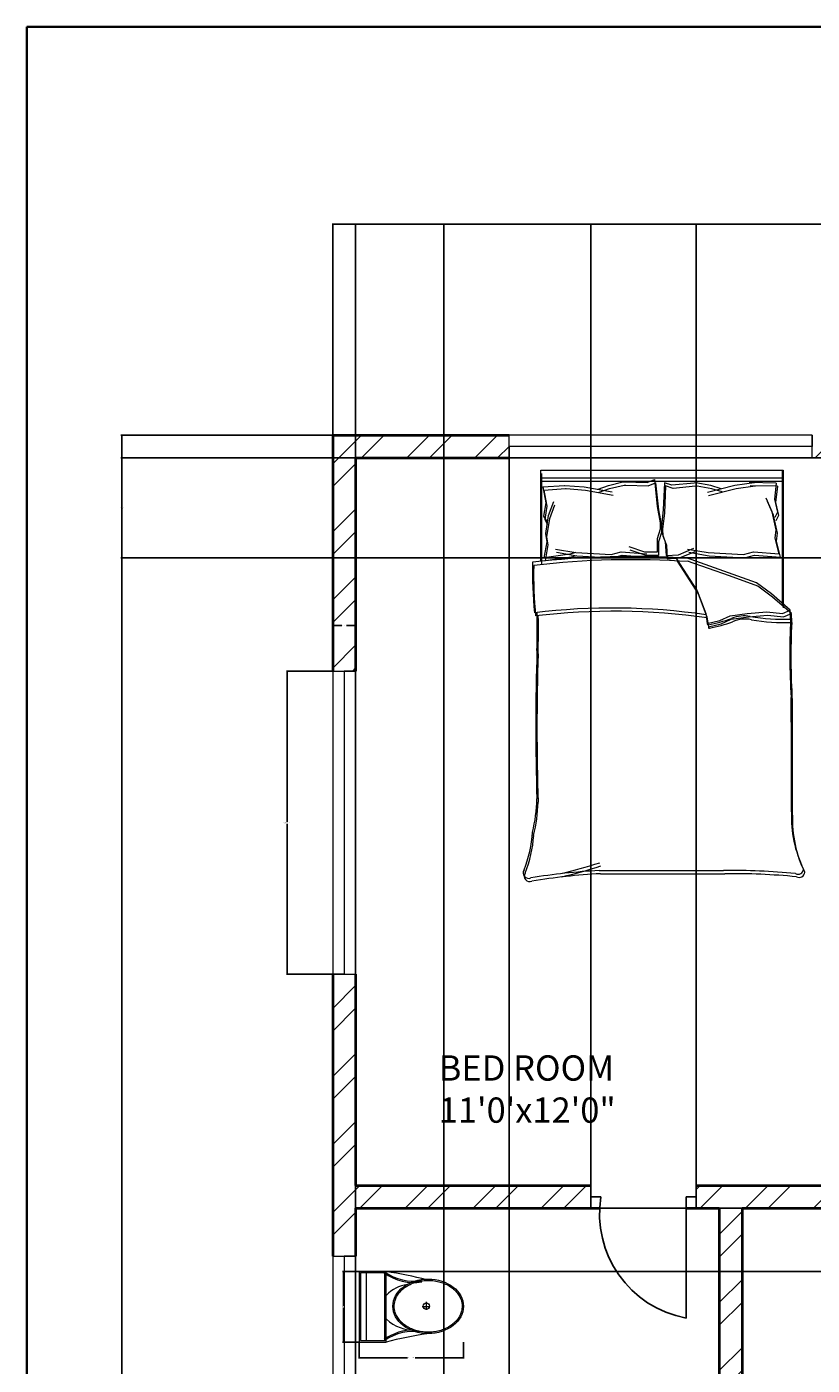
# Model space of a CAD drawing. Units: inches. Extents: x 2063 to 2617, y 1299 to 2210.
# Tile 13 of 22: x 2063 to 2218, y 1945 to 2210. Entities that reach past the tile are written whole.
import ezdxf

# ---------------------------------------------------------------- set-up
doc = ezdxf.new("R2010")
doc.units = ezdxf.units.IN
for name, color, linetype, lineweight in [('A-ANNO-DIMS', 2, 'Continuous', 18), ('A-ANNO-TTLB', 7, 'Continuous', 35), ('A-AREA-IDEN', 7, 'Continuous', 18), ('A-DOOR', 11, 'Continuous', 25), ('A-FLOR-FIXT', 8, 'Continuous', 18), ('A-FURN', 8, 'Continuous', 18), ('A-GLAZ', 123, 'Continuous', 18), ('A-WALL', 7, 'Continuous', 40)]:
    doc.layers.add(name, color=color, linetype=linetype, lineweight=lineweight)
doc.layers.add('A-WALL-PATT', color=215, linetype='Continuous', lineweight=13, true_color=0xa953a0)
doc.styles.get("Standard").update_dxf_attribs({"font": 'arial.ttf'})
doc.dimstyles.get("Standard").update_dxf_attribs({"dimtxt": 0.18, "dimasz": 0.18, "dimexe": 0.18, "dimexo": 0.0625, "dimgap": 0.09, "dimtad": 0, "dimtih": 1, "dimtoh": 1, "dimdec": 4, "dimzin": 0, "dimdsep": 46, "dimtxsty": 'Standard', "dimcen": 0.09, "dimadec": 0, "dimazin": 0, "dimtfac": 1, "dimtdec": 4, "dimtofl": 0, "dimtmove": 0, "dimatfit": 3, "dimfxl": 1, "dimtolj": 1, "dimtzin": 0, "dimarcsym": 0})

# ---------------------------------------------------------------- blocks, each defined once
blk = doc.blocks.new('A$C31115884')
for p, q in [((283.1, 497.7), (223.4, 497.7)), ((257.5, 466.4), (257.5, 523.2)), ((0, 200), (0, 0)), ((520, 200), (0, 200)), ((520, 0), (520, 200)), ((10, 190), (10, 10)), ((510, 190), (10, 190)), ((510, 10), (510, 190)), ((510, 54.5), (0, 54.5)), ((10, 10), (510, 10)), ((0, 0), (520, 0))]:
    blk.add_line(p, q)
blk.add_circle((255.6, 496.4), 23.6)
for centre, radius, start, end in [((2777.7, -204.6), 2807, 165.4549, 171.71327), ((3237, 905), 2807, 188.28673, 194.5451), ((-294.5, 403.3), 364.7, 324.20913, 9.34987), ((-294.5, 403.3), 374.7, 324.20913, 9.34987), ((139.5, 406.2), 293.5, 315.84364, 2.65635), ((805.8, 403.3), 374.7, 179.20365, 215.79087), ((805.8, 403.3), 364.7, 170.65013, 215.79087), ((383.6, 406.2), 293.5, 190.27735, 224.15636)]:
    blk.add_arc(centre, radius, start, end)
blk.add_ellipse((256.2, 509.9), major_axis=(0, -260.7), ratio=0.772727)
blk.add_open_spline([(256.2, 259.2), (263.1, 259.2), (270, 259.7), (287.8, 262.3), (298.7, 265.1), (319.9, 273.1), (330.2, 278.4), (350.1, 291.1), (359.7, 298.7), (377.7, 315.9), (386.2, 325.5), (401.7, 346.6), (408.8, 358.1), (421.3, 382.5), (426.8, 395.5), (435.9, 422.4), (439.5, 436.4), (444.8, 465.1), (446.5, 479.7), (447.9, 509.2), (447.6, 524), (445, 553.3), (442.7, 567.8), (436.3, 596), (432.1, 609.7), (421.9, 636), (416, 648.6), (402.5, 672.1), (395, 683), (378.6, 703), (369.8, 712.1), (351.1, 728), (341.3, 734.8), (320.9, 746.2), (310.4, 750.7), (288.9, 757.3), (278, 759.4), (256, 761), (245, 760.6), (223.1, 757.2), (212.3, 754.3), (191.1, 746.1), (180.8, 740.7), (160.9, 727.8), (151.4, 720.1), (133.5, 702.7), (125.1, 693), (109.6, 671.7), (102.6, 660.2), (90.2, 635.7), (84.9, 622.7), (76, 595.6), (72.4, 581.6), (67.2, 552.9), (65.6, 538.2), (64.4, 508.8), (64.8, 494), (67.5, 464.7), (69.9, 450.2), (76.6, 422), (80.8, 408.3), (91.1, 382.2), (97.2, 369.7), (110.8, 346.3), (118.4, 335.4), (134.8, 315.6), (143.7, 306.7), (162.4, 290.9), (172.3, 284.2), (192.8, 273), (203.3, 268.6), (224.8, 262.2), (235.8, 260.2), (249.9, 259.3), (253, 259.2), (256.2, 259.2)], degree=3, knots=[0, 0, 0, 0, 0.110105, 0.110105, 0.285049, 0.285049, 0.459994, 0.459994, 0.634938, 0.634938, 0.809882, 0.809882, 0.984827, 0.984827, 1.159771, 1.159771, 1.334715, 1.334715, 1.50966, 1.50966, 1.684604, 1.684604, 1.859549, 1.859549, 2.034493, 2.034493, 2.209437, 2.209437, 2.384382, 2.384382, 2.559326, 2.559326, 2.73427, 2.73427, 2.909215, 2.909215, 3.084159, 3.084159, 3.259103, 3.259103, 3.434048, 3.434048, 3.608992, 3.608992, 3.783936, 3.783936, 3.958881, 3.958881, 4.133825, 4.133825, 4.30877, 4.30877, 4.483714, 4.483714, 4.658658, 4.658658, 4.833603, 4.833603, 5.008547, 5.008547, 5.183491, 5.183491, 5.358436, 5.358436, 5.53338, 5.53338, 5.708324, 5.708324, 5.883269, 5.883269, 6.058213, 6.058213, 6.233158, 6.233158, 6.283185, 6.283185, 6.283185, 6.283185])
blk = doc.blocks.new('BED-DOUBLE')
for p, q in [((3.48, 63.33), (3.48, 81.44)), ((3.48, 63.33), (3.48, 81.44)), ((3.48, 81.44), (51.49, 81.44)), ((3.48, 79.91), (51.27, 79.91)), ((3.48, 79.91), (51.27, 79.91)), ((3.7, 62.69), (3.7, 80.8)), ((3.7, 62.69), (3.7, 80.8)), ((24.54, 79), (25.98, 79.57)), ((24.54, 79), (25.98, 79.57)), ((25.98, 79.57), (26.56, 74.22)), ((25.98, 79.57), (26.56, 74.22)), ((51.27, 81.44), (51.27, 54.83)), ((51.27, 81.44), (51.27, 54.83)), ((51.49, 81.44), (51.49, 80.8)), ((51.49, 80.8), (51.49, 54.19)), ((51.49, 80.8), (51.49, 54.19)), ((3.7, 79.27), (51.49, 79.27)), ((3.7, 79.27), (51.49, 79.27)), ((3.89, 78.13), (4.47, 74.95)), ((3.9, 78.11), (8.18, 78.43)), ((3.9, 78.11), (8.18, 78.43)), ((3.9, 78.13), (4.47, 74.95)), ((4.12, 77.49), (4.7, 74.31)), ((4.12, 77.49), (4.7, 74.31)), ((4.13, 77.47), (8.41, 77.8)), ((4.13, 77.47), (8.41, 77.8)), ((8.18, 78.43), (8.29, 78.42)), ((8.18, 78.43), (8.29, 78.42)), ((8.29, 78.42), (12.11, 78.13)), ((8.29, 78.42), (12.11, 78.13)), ((8.41, 77.8), (8.51, 77.78)), ((8.41, 77.8), (8.51, 77.78)), ((8.51, 77.78), (12.34, 77.49)), ((8.51, 77.78), (12.34, 77.49)), ((12.11, 78.13), (17.6, 77.12)), ((12.11, 78.13), (17.6, 77.12)), ((12.34, 77.49), (17.83, 76.48)), ((12.34, 77.49), (17.83, 76.48)), ((14.86, 77.69), (16.88, 78.42)), ((14.86, 77.69), (16.88, 78.42)), ((15.08, 77.05), (17.11, 77.78)), ((15.08, 77.05), (17.11, 77.78)), ((16.88, 78.42), (19.77, 79.14)), ((16.88, 78.42), (19.77, 79.14)), ((17.11, 77.78), (20, 78.5)), ((17.11, 77.78), (20, 78.5)), ((19.77, 79.14), (20.09, 79.14)), ((19.77, 79.14), (20.09, 79.14)), ((20, 78.5), (20.32, 78.5)), ((20, 78.5), (20.32, 78.5)), ((20.09, 79.14), (24.54, 79)), ((20.09, 79.14), (24.54, 79)), ((20.32, 78.5), (24.77, 78.36)), ((20.32, 78.5), (24.77, 78.36)), ((24.77, 78.36), (26.21, 78.93)), ((24.77, 78.36), (26.21, 78.93)), ((26.21, 78.93), (26.79, 73.58)), ((26.21, 78.93), (26.79, 73.58)), ((27.98, 78.95), (27.73, 73.58)), ((27.98, 78.95), (27.73, 73.58)), ((28.21, 78.31), (27.96, 72.94)), ((28.21, 78.31), (27.96, 72.94)), ((29.46, 78.46), (27.98, 78.95)), ((29.46, 78.46), (27.98, 78.95)), ((29.68, 77.83), (28.21, 78.31)), ((29.68, 77.83), (28.21, 78.31)), ((33.88, 78.89), (29.46, 78.46)), ((33.88, 78.89), (29.46, 78.46)), ((34.11, 78.25), (29.68, 77.83)), ((34.11, 78.25), (29.68, 77.83)), ((34.21, 78.91), (33.88, 78.89)), ((34.2, 78.91), (33.88, 78.89)), ((34.43, 78.27), (34.11, 78.25)), ((34.43, 78.27), (34.11, 78.25)), ((37.14, 78.37), (34.2, 78.91)), ((37.14, 78.37), (34.21, 78.91)), ((37.36, 77.73), (34.43, 78.27)), ((37.36, 77.73), (34.43, 78.27)), ((41.91, 78.37), (36.5, 77.02)), ((41.91, 78.37), (36.5, 77.02)), ((42.14, 77.73), (36.72, 76.38)), ((42.14, 77.73), (36.72, 76.38)), ((39.2, 77.77), (37.14, 78.37)), ((39.2, 77.77), (37.14, 78.37)), ((39.43, 77.13), (37.36, 77.73)), ((39.43, 77.13), (37.36, 77.73)), ((45.71, 78.9), (41.91, 78.37)), ((45.71, 78.9), (41.91, 78.37)), ((45.94, 78.26), (42.14, 77.73)), ((45.94, 78.26), (42.14, 77.73)), ((50.11, 78.89), (44.71, 78.98)), ((44.71, 78.98), (45.71, 78.9)), ((50.11, 78.89), (44.71, 78.98)), ((44.71, 78.98), (45.71, 78.9)), ((50.34, 78.25), (44.94, 78.34)), ((44.94, 78.34), (45.94, 78.26)), ((50.34, 78.25), (44.94, 78.34)), ((44.94, 78.34), (45.94, 78.26)), ((50.11, 78.89), (49.73, 75.68)), ((50.11, 78.89), (49.73, 75.68)), ((50.34, 78.25), (49.96, 75.04)), ((50.34, 78.25), (49.96, 75.04)), ((4.47, 74.95), (4.04, 72.34)), ((4.47, 74.95), (4.04, 72.34)), ((4.7, 74.31), (4.27, 71.7)), ((4.7, 74.31), (4.27, 71.7)), ((5.05, 72.49), (6.06, 75.24)), ((5.05, 72.49), (6.06, 75.24)), ((5.28, 71.85), (6.29, 74.6)), ((5.28, 71.85), (6.29, 74.6)), ((26.56, 74.22), (27.14, 71.04)), ((26.56, 74.22), (27.14, 71.04)), ((49.31, 73.19), (48.13, 75.87)), ((49.31, 73.19), (48.13, 75.87)), ((49.54, 72.55), (48.36, 75.23)), ((49.54, 72.55), (48.36, 75.23)), ((49.73, 75.68), (50.33, 73.11)), ((49.73, 75.68), (50.33, 73.11)), ((49.96, 75.04), (50.56, 72.47)), ((49.96, 75.04), (50.56, 72.47)), ((4.04, 72.34), (4.62, 71.33)), ((4.04, 72.34), (4.62, 71.33)), ((4.27, 71.7), (4.85, 70.69)), ((4.27, 71.7), (4.85, 70.69)), ((4.47, 68.87), (5.05, 72.49)), ((4.47, 68.87), (5.05, 72.49)), ((4.7, 68.23), (5.28, 71.85)), ((4.7, 68.23), (5.28, 71.85)), ((26.79, 73.58), (27.37, 70.4)), ((26.79, 73.58), (27.37, 70.4)), ((27.73, 73.58), (27.36, 70.37)), ((27.73, 73.58), (27.36, 70.37)), ((27.96, 72.94), (27.58, 69.73)), ((27.96, 72.94), (27.58, 69.73)), ((50.11, 69.61), (49.31, 73.19)), ((50.11, 69.61), (49.31, 73.19)), ((50.34, 68.98), (49.54, 72.55)), ((50.34, 68.98), (49.54, 72.55)), ((50.33, 73.11), (49.81, 72.06)), ((50.33, 73.11), (49.82, 72.06)), ((50.56, 72.47), (50.04, 71.42)), ((50.56, 72.47), (50.04, 71.42)), ((27.14, 69.74), (26.56, 67.86)), ((27.14, 69.74), (26.56, 67.86)), ((27.37, 69.1), (26.79, 67.22)), ((27.37, 69.1), (26.79, 67.22)), ((27.14, 71.04), (27.14, 69.74)), ((27.14, 71.04), (27.14, 69.74)), ((27.36, 70.37), (27.44, 69.07)), ((27.36, 70.37), (27.44, 69.07)), ((27.37, 70.4), (27.37, 69.1)), ((27.37, 70.4), (27.37, 69.1)), ((27.44, 69.07), (28.13, 67.23)), ((27.44, 69.07), (28.13, 67.23)), ((27.58, 69.73), (27.66, 68.43)), ((27.58, 69.73), (27.66, 68.43)), ((49.92, 68.01), (50.11, 69.61)), ((49.92, 68.01), (50.11, 69.61)), ((50.15, 67.37), (50.34, 68.98)), ((50.15, 67.37), (50.34, 68.98)), ((4.18, 64.1), (4.76, 67.28)), ((4.18, 64.1), (4.76, 67.28)), ((4.41, 63.46), (4.99, 66.64)), ((4.41, 63.46), (4.99, 66.64)), ((4.76, 67.28), (4.47, 68.87)), ((4.76, 67.28), (4.47, 68.87)), ((4.99, 66.64), (4.7, 68.23)), ((4.99, 66.64), (4.7, 68.23)), ((24.1, 65.18), (20.96, 66.27)), ((24.1, 65.18), (20.96, 66.27)), ((26.56, 67.86), (26.56, 65.18)), ((26.56, 67.86), (26.56, 65.18)), ((26.79, 67.22), (26.79, 64.54)), ((26.79, 67.22), (26.79, 64.54)), ((27.66, 68.43), (28.36, 66.59)), ((27.66, 68.43), (28.36, 66.59)), ((28.13, 67.23), (28.3, 64.55)), ((28.13, 67.23), (28.3, 64.55)), ((28.36, 66.59), (28.53, 63.91)), ((28.36, 66.59), (28.53, 63.91)), ((50.7, 64.87), (49.92, 68.01)), ((50.7, 64.87), (49.92, 68.01)), ((50.93, 64.23), (50.15, 67.37)), ((50.93, 64.23), (50.15, 67.37)), ((9.28, 64.83), (4.18, 64.1)), ((9.28, 64.83), (4.18, 64.1)), ((9.51, 64.19), (4.41, 63.46)), ((9.51, 64.19), (4.41, 63.46)), ((6.38, 65.82), (10.41, 65.15)), ((6.38, 65.82), (10.41, 65.15)), ((6.61, 65.18), (10.64, 64.51)), ((6.61, 65.18), (10.64, 64.51)), ((10.41, 65.15), (9.28, 64.83)), ((10.41, 65.15), (9.28, 64.83)), ((10.64, 64.51), (9.51, 64.19)), ((10.64, 64.51), (9.51, 64.19)), ((10.41, 65.15), (17.42, 64.72)), ((10.41, 65.15), (17.42, 64.72)), ((10.64, 64.51), (17.65, 64.08)), ((10.64, 64.51), (17.65, 64.08)), ((17.42, 64.72), (19.38, 65.27)), ((17.42, 64.72), (19.38, 65.27)), ((17.65, 64.08), (19.61, 64.64)), ((17.65, 64.08), (19.61, 64.64)), ((19.38, 65.27), (24.52, 64.87)), ((19.38, 65.27), (24.52, 64.87)), ((19.61, 64.64), (24.74, 64.23)), ((19.61, 64.64), (24.74, 64.23)), ((24.33, 64.54), (21.19, 65.63)), ((24.33, 64.54), (21.19, 65.63)), ((26.56, 65.18), (24.1, 65.18)), ((26.56, 65.18), (24.1, 65.18)), ((26.79, 64.54), (24.33, 64.54)), ((26.79, 64.54), (24.33, 64.54)), ((28.3, 64.55), (30.75, 64.7)), ((28.3, 64.55), (30.75, 64.7)), ((28.53, 63.91), (30.98, 64.06)), ((28.53, 63.91), (30.98, 64.06)), ((30.26, 64.06), (34.45, 57.57)), ((30.26, 64.06), (34.45, 57.57)), ((30.75, 64.7), (33.82, 65.99)), ((30.75, 64.7), (33.82, 65.99)), ((30.98, 64.06), (34.05, 65.35)), ((30.98, 64.06), (34.05, 65.35)), ((40.64, 61.13), (32.31, 64.06)), ((40.64, 61.13), (32.31, 64.06)), ((32.56, 65.82), (36.6, 65.15)), ((32.56, 65.82), (36.6, 65.15)), ((32.79, 65.18), (36.83, 64.51)), ((32.79, 65.18), (36.82, 64.51)), ((36.6, 65.15), (43.61, 64.72)), ((36.6, 65.15), (43.61, 64.72)), ((36.82, 64.51), (43.83, 64.08)), ((36.83, 64.51), (43.84, 64.08)), ((43.61, 64.72), (45.57, 65.27)), ((43.61, 64.72), (45.57, 65.27)), ((43.83, 64.08), (45.8, 64.64)), ((43.84, 64.08), (45.8, 64.64)), ((45.57, 65.27), (50.7, 64.87)), ((45.57, 65.27), (50.7, 64.87)), ((45.8, 64.64), (50.93, 64.23)), ((45.8, 64.64), (50.93, 64.23)), ((30.49, 63.42), (34.68, 56.93)), ((30.49, 63.42), (34.68, 56.93)), ((40.87, 60.49), (32.53, 63.42)), ((40.87, 60.49), (32.54, 63.42)), ((46.22, 59.11), (40.64, 61.13)), ((46.22, 59.11), (40.64, 61.13)), ((46.45, 58.48), (40.87, 60.49)), ((46.45, 58.48), (40.87, 60.49)), ((49.16, 56.95), (46.22, 59.11)), ((49.16, 56.95), (46.22, 59.11)), ((49.39, 56.31), (46.45, 58.48)), ((49.39, 56.31), (46.45, 58.48)), ((34.45, 57.57), (36.15, 53.08)), ((34.45, 57.57), (36.15, 53.08)), ((34.68, 56.93), (36.38, 52.44)), ((34.68, 56.93), (36.38, 52.44)), ((52.87, 53.7), (49.16, 56.95)), ((52.87, 53.7), (49.16, 56.95)), ((53.1, 53.06), (49.39, 56.31)), ((53.1, 53.06), (49.39, 56.31)), ((36.15, 53.08), (36.46, 51.07)), ((36.15, 53.08), (36.46, 51.07)), ((40.95, 52.61), (44.36, 53.08)), ((40.95, 52.61), (44.36, 53.08)), ((44.36, 53.08), (48.23, 53.39)), ((44.36, 53.08), (48.23, 53.39)), ((48.23, 53.39), (51.33, 53.08)), ((48.23, 53.39), (51.33, 53.08)), ((51.33, 53.08), (52.87, 53.7)), ((51.33, 53.08), (52.87, 53.7)), ((51.56, 52.44), (53.1, 53.06)), ((51.56, 52.44), (53.1, 53.06)), ((52.95, 51.95), (52.87, 53.7, 3.87)), ((52.95, 51.95), (52.87, 53.7, 3.87)), ((53.18, 51.31), (53.1, 53.06, 3.87)), ((53.18, 51.31), (53.1, 53.06, 3.87)), ((36.38, 52.44), (36.69, 50.43)), ((36.38, 52.44), (36.69, 50.43)), ((36.46, 51.07), (38.94, 51.69)), ((36.46, 51.07), (38.94, 51.69)), ((36.69, 50.43), (39.17, 51.05)), ((36.69, 50.43), (39.17, 51.05)), ((38.94, 51.69), (40.95, 52.61)), ((38.94, 51.69), (40.95, 52.61)), ((39.17, 51.05), (41.18, 51.97)), ((39.17, 51.05), (41.18, 51.97)), ((41.18, 51.97), (44.59, 52.44)), ((41.18, 51.97), (44.59, 52.44)), ((44.59, 52.44), (48.46, 52.75)), ((44.59, 52.44), (48.46, 52.75)), ((48.46, 52.75), (51.56, 52.44)), ((48.46, 52.75), (51.56, 52.44)), ((15.06, 2.2), (39.68, 2.2)), ((15.06, 2.2), (39.68, 2.2)), ((15.29, 1.56), (39.91, 1.56)), ((15.29, 1.56), (39.91, 1.56))]:
    blk.add_line(p, q)
for centre, radius, start, end in [((21.36, -100.61), 164.97, 86.0865, 96.7821), ((21.36, -100.61), 164.97, 86.0865, 96.7821), ((21.59, -101.25), 164.97, 86.0865, 96.7821), ((21.59, -101.25), 164.97, 86.0865, 96.7821), ((85.16, 61.35), 83.31, 178.7218, 185.604), ((85.16, 61.35), 83.31, 178.7218, 185.604), ((85.39, 60.71), 83.31, 178.7218, 185.604), ((85.39, 60.71), 83.31, 178.7218, 185.604), ((17.76, -74.87), 129.02, 81.7845, 96.9006), ((17.76, -74.87), 129.02, 81.7845, 96.9006), ((17.98, -75.51), 129.02, 81.7845, 96.9006), ((17.98, -75.51), 129.02, 81.7845, 96.9006), ((-167.31, 50.27), 170.11, 358.4762, 1.0082), ((-167.31, 50.27), 170.11, 358.4762, 1.0082), ((-167.08, 49.63), 170.11, 358.4762, 1.0082), ((-167.08, 49.63), 170.11, 358.4762, 1.0082), ((36.64, 51), 0.185, 160.2464, 271.1377), ((36.64, 51), 0.185, 160.2464, 271.1377), ((31.15, 79.96), 29.65, 280.6617, 289.8806), ((31.15, 79.96), 29.65, 280.6617, 289.8806), ((36.87, 50.36), 0.185, 160.2464, 271.1377), ((36.86, 50.36), 0.185, 160.2464, 271.1377), ((31.38, 79.32), 29.65, 280.6617, 289.8806), ((31.38, 79.32), 29.65, 280.6617, 289.8806), ((43.74, 46.38), 6.22, 78.6608, 113.7384), ((43.74, 46.38), 6.22, 78.6608, 113.7384), ((43.97, 45.74), 6.22, 78.6608, 113.7384), ((43.97, 45.74), 6.22, 78.6608, 113.7384), ((51.33, 88.1), 36.18, 259.8763, 272.5657), ((51.33, 88.1), 36.18, 259.8763, 272.5657), ((51.56, 87.46), 36.18, 259.8763, 272.5657), ((51.56, 87.46), 36.18, 259.8763, 272.5657), ((182.27, 45.13), 129.5, 176.9791, 183.8365), ((182.27, 45.13), 129.5, 176.9791, 183.8365), ((182.49, 44.49), 129.5, 176.9791, 183.8365), ((182.49, 44.49), 129.5, 176.9791, 183.8365), ((484.82, 30.83), 482.31, 178.2277, 181.7185), ((484.82, 30.83), 482.31, 178.2277, 181.7185), ((485.05, 30.19), 482.31, 178.2277, 181.7185), ((485.05, 30.19), 482.31, 178.2277, 181.7185), ((-4508.74, 13.62), 4561.86, 0.00217, 0.28689), ((-4508.74, 13.62), 4561.86, 0.00217, 0.28689), ((-4508.51, 12.98), 4561.86, 0.00217, 0.28689), ((-4508.51, 12.98), 4561.86, 0.00217, 0.28689), ((-26.9, 16.93), 29.63, 346.0648, 358.9113), ((-26.9, 16.93), 29.63, 346.0648, 358.9113), ((-26.67, 16.29), 29.63, 346.0648, 358.9113), ((-26.67, 16.29), 29.63, 346.0648, 358.9113), ((76.16, 12.78), 23.07, 177.4714, 206.4681), ((76.16, 12.78), 23.07, 177.4714, 206.4681), ((76.39, 12.14), 23.07, 177.4714, 206.4681), ((76.39, 12.14), 23.07, 177.4714, 206.4681), ((-21.66, 11.17), 23.56, 337.9751, 356.652), ((-21.66, 11.17), 23.56, 337.9751, 356.652), ((-21.43, 10.53), 23.56, 337.9751, 356.652), ((-21.43, 10.53), 23.56, 337.9751, 356.652), ((-17.22, 105.16), 106.46, 283.3832, 287.7053), ((-17.22, 105.16), 106.46, 283.3832, 287.7053), ((-16.99, 104.52), 106.46, 283.3832, 287.7053), ((-16.99, 104.52), 106.46, 283.3832, 287.7053), ((1.09, 1.73), 1.09, 146.1736, 293.4781), ((1.09, 1.73), 1.09, 146.1736, 293.4781), ((1.32, 1.09), 1.09, 146.1736, 293.4781), ((1.32, 1.09), 1.09, 146.1736, 293.4781), ((21.43, -119.39), 121.76, 92.9958, 99.4091), ((21.43, -119.39), 121.76, 92.9958, 99.4091), ((21.66, -120.03), 121.76, 92.9958, 99.4091), ((21.66, -120.03), 121.76, 92.9958, 99.4091), ((41.15, -130.83), 133.04, 84.4998, 90.6351), ((41.15, -130.83), 133.04, 84.4998, 90.6351), ((41.38, -131.47), 133.04, 84.4998, 90.6351), ((41.38, -131.47), 133.04, 84.4998, 90.6351), ((54.41, 2.57), 1.1, 242.6588, 356.02), ((54.41, 2.57), 1.1, 242.6588, 356.02), ((54.64, 1.93), 1.1, 242.6588, 356.02), ((54.64, 1.93), 1.1, 242.6588, 356.02)]:
    blk.add_arc(centre, radius, start, end)
blk = doc.blocks.new('WIN-60IN')
for p, q in [((0, 60), (4.5, 60)), ((0, 60), (0, 0)), ((4.5, 60), (2.25, 60)), ((2.25, 60), (2.25, 0)), ((4.5, 60), (4.5, 0)), ((2.25, 0), (0, 0)), ((0, 0), (4.5, 0))]:
    blk.add_line(p, q)
blk = doc.blocks.new('WIN-24IN')
for p, q in [((0, 24), (4.5, 24)), ((0, 24), (0, 0)), ((4.5, 24), (2.25, 24)), ((2.25, 24), (2.25, 0)), ((4.5, 24), (4.5, 0)), ((2.25, 0), (0, 0)), ((0, 0), (4.5, 0))]:
    blk.add_line(p, q)
blk = doc.blocks.new('*D11')
at = {"layer": 'A-ANNO-DIMS', "color": 0, "lineweight": -2, "transparency": 16777216}
for p, q in [((2123.08, 2082.12), (2113.96, 2082.12)), ((2114.14, 2081.94), (2114.14, 2052.3)), ((2114.14, 2022.3), (2114.14, 2051.93)), ((2123.08, 2022.12), (2113.96, 2022.12))]:
    blk.add_line(p, q, dxfattribs=at)
at = {"layer": 'A-ANNO-DIMS', "color": 0, "transparency": 16777216}
for points in [[(2114.11, 2081.94), (2114.17, 2081.94), (2114.14, 2082.12)], [(2114.11, 2022.3), (2114.17, 2022.3), (2114.14, 2022.12)]]:
    blk.add_solid(points, dxfattribs=at)
at = {"layer": 'Defpoints', "color": 0, "transparency": 16777216}
for p in [(2114.14, 2082.12), (2123.14, 2082.12), (2123.14, 2022.12)]:
    blk.add_point(p, dxfattribs=at)
at = {"layer": 'A-ANNO-DIMS', "color": 0, "transparency": 16777216, "insert": (2114.14, 2052.12), "char_height": 0.18, "attachment_point": 5}
blk.add_mtext('\\A1;WIN. 60 TYP.', dxfattribs=at)
blk = doc.blocks.new('*D12')
at = {"layer": 'A-ANNO-DIMS', "color": 0, "lineweight": -2, "transparency": 16777216}
for p, q in [((2123.14, 2082.18), (2123.14, 2091.3)), ((2123.32, 2091.12), (2124.94, 2091.12)), ((2127.46, 2091.12), (2125.85, 2091.12)), ((2127.64, 2082.18), (2127.64, 2091.3))]:
    blk.add_line(p, q, dxfattribs=at)
at = {"layer": 'A-ANNO-DIMS', "color": 0, "transparency": 16777216}
for points in [[(2123.32, 2091.15), (2123.32, 2091.09), (2123.14, 2091.12)], [(2127.46, 2091.15), (2127.46, 2091.09), (2127.64, 2091.12)]]:
    blk.add_solid(points, dxfattribs=at)
at = {"layer": 'Defpoints', "color": 0, "transparency": 16777216}
for p in [(2127.64, 2091.12), (2123.14, 2082.12), (2127.64, 2082.12)]:
    blk.add_point(p, dxfattribs=at)
at = {"layer": 'A-ANNO-DIMS', "color": 0, "transparency": 16777216, "insert": (2125.39, 2091.12), "char_height": 0.18, "attachment_point": 5}
blk.add_mtext('\\A1;5 TYP.', dxfattribs=at)
blk = doc.blocks.new('*D15')
at = {"layer": 'A-ANNO-DIMS', "color": 0, "lineweight": -2, "transparency": 16777216}
for p, q in [((2128.36, 1949.28), (2128.36, 1946.06)), ((2149.01, 1949.28), (2149.01, 1946.06)), ((2128.54, 1946.24), (2137.91, 1946.24)), ((2148.83, 1946.24), (2139.46, 1946.24))]:
    blk.add_line(p, q, dxfattribs=at)
at = {"layer": 'A-ANNO-DIMS', "color": 0, "transparency": 16777216}
for points in [[(2128.54, 1946.27), (2128.54, 1946.21), (2128.36, 1946.24)], [(2148.83, 1946.27), (2148.83, 1946.21), (2149.01, 1946.24)]]:
    blk.add_solid(points, dxfattribs=at)
at = {"layer": 'Defpoints', "color": 0, "transparency": 16777216}
for p in [(2128.36, 1949.34), (2149.01, 1949.34), (2149.01, 1946.24)]:
    blk.add_point(p, dxfattribs=at)
at = {"layer": 'A-ANNO-DIMS', "color": 0, "transparency": 16777216, "insert": (2138.68, 1946.24), "char_height": 0.18, "attachment_point": 5}
blk.add_mtext('\\A1;WC 21 TYP.', dxfattribs=at)
blk = doc.blocks.new('*D16')
at = {"layer": 'A-ANNO-DIMS', "color": 0, "lineweight": -2, "transparency": 16777216}
for p, q in [((2128.3, 1963.28), (2125.08, 1963.28)), ((2125.26, 1963.1), (2125.26, 1956.49)), ((2125.26, 1949.52), (2125.26, 1956.13)), ((2128.3, 1949.34), (2125.08, 1949.34))]:
    blk.add_line(p, q, dxfattribs=at)
at = {"layer": 'A-ANNO-DIMS', "color": 0, "transparency": 16777216}
for points in [[(2125.23, 1963.1), (2125.29, 1963.1), (2125.26, 1963.28)], [(2125.23, 1949.52), (2125.29, 1949.52), (2125.26, 1949.34)]]:
    blk.add_solid(points, dxfattribs=at)
at = {"layer": 'Defpoints', "color": 0, "transparency": 16777216}
for p in [(2128.36, 1963.28), (2125.26, 1949.34), (2128.36, 1949.34)]:
    blk.add_point(p, dxfattribs=at)
at = {"layer": 'A-ANNO-DIMS', "color": 0, "transparency": 16777216, "insert": (2125.26, 1956.31), "char_height": 0.18, "attachment_point": 5}
blk.add_mtext('\\A1;14 TYP.', dxfattribs=at)
blk = doc.blocks.new('*D31')
at = {"layer": 'A-ANNO-DIMS', "color": 0, "lineweight": -2, "transparency": 16777216}
for p, q in [((2123.14, 2128.87), (2123.14, 2170.74)), ((2123.32, 2170.56), (2338, 2170.56)), ((2553.46, 2170.56), (2338.79, 2170.56)), ((2553.64, 2128.87), (2553.64, 2170.74))]:
    blk.add_line(p, q, dxfattribs=at)
at = {"layer": 'A-ANNO-DIMS', "color": 0, "transparency": 16777216}
for points in [[(2123.32, 2170.59), (2123.32, 2170.53), (2123.14, 2170.56)], [(2553.46, 2170.59), (2553.46, 2170.53), (2553.64, 2170.56)]]:
    blk.add_solid(points, dxfattribs=at)
at = {"layer": 'Defpoints', "color": 0, "transparency": 16777216}
for p in [(2553.64, 2170.56), (2123.14, 2128.81), (2553.64, 2128.81)]:
    blk.add_point(p, dxfattribs=at)
at = {"layer": 'A-ANNO-DIMS', "color": 0, "transparency": 16777216, "insert": (2338.39, 2170.56), "char_height": 0.18, "attachment_point": 5}
blk.add_mtext('\\A1;430.5', dxfattribs=at)
blk = doc.blocks.new('*D32')
at = {"layer": 'A-ANNO-DIMS', "color": 0, "lineweight": -2, "transparency": 16777216}
for p, q in [((2123.08, 2128.81), (2081.21, 2128.81)), ((2081.39, 2128.63), (2081.39, 1765.49)), ((2081.39, 1401.99), (2081.39, 1765.13)), ((2123.08, 1401.81), (2081.21, 1401.81))]:
    blk.add_line(p, q, dxfattribs=at)
at = {"layer": 'A-ANNO-DIMS', "color": 0, "transparency": 16777216}
for points in [[(2081.36, 2128.63), (2081.42, 2128.63), (2081.39, 2128.81)], [(2081.36, 1401.99), (2081.42, 1401.99), (2081.39, 1401.81)]]:
    blk.add_solid(points, dxfattribs=at)
at = {"layer": 'Defpoints', "color": 0, "transparency": 16777216}
for p in [(2081.39, 2128.81), (2123.14, 2128.81), (2123.14, 1401.81)]:
    blk.add_point(p, dxfattribs=at)
at = {"layer": 'A-ANNO-DIMS', "color": 0, "transparency": 16777216, "insert": (2081.39, 1765.31), "char_height": 0.18, "attachment_point": 5}
blk.add_mtext('\\A1;727', dxfattribs=at)
blk = doc.blocks.new('*D49')
at = {"layer": 'A-ANNO-DIMS', "color": 0, "lineweight": -2, "transparency": 16777216}
for p, q in [((2127.64, 2124.25), (2127.64, 1317.7)), ((2158.04, 2124.25), (2158.04, 1317.7)), ((2127.82, 1317.88), (2142.38, 1317.88)), ((2157.86, 1317.88), (2143.31, 1317.88))]:
    blk.add_line(p, q, dxfattribs=at)
at = {"layer": 'A-ANNO-DIMS', "color": 0, "transparency": 16777216}
for points in [[(2127.82, 1317.91), (2127.82, 1317.85), (2127.64, 1317.88)], [(2157.86, 1317.91), (2157.86, 1317.85), (2158.04, 1317.88)]]:
    blk.add_solid(points, dxfattribs=at)
at = {"layer": 'Defpoints', "color": 0, "transparency": 16777216}
for p in [(2127.64, 2124.31), (2158.04, 2124.31), (2158.04, 1317.88)]:
    blk.add_point(p, dxfattribs=at)
at = {"layer": 'A-ANNO-DIMS', "color": 0, "transparency": 16777216, "insert": (2142.84, 1317.88), "char_height": 0.18, "attachment_point": 5}
blk.add_mtext('\\A1;30.396', dxfattribs=at)
blk = doc.blocks.new('*D53')
at = {"layer": 'A-ANNO-DIMS', "color": 0, "lineweight": -2, "transparency": 16777216}
for p, q in [((2412.58, 2124.31), (2081.21, 2124.31)), ((2081.39, 2124.13), (2081.39, 2114.6)), ((2081.39, 2104.7), (2081.39, 2114.23)), ((2412.58, 2104.52), (2081.21, 2104.52))]:
    blk.add_line(p, q, dxfattribs=at)
at = {"layer": 'A-ANNO-DIMS', "color": 0, "transparency": 16777216}
for points in [[(2081.36, 2124.13), (2081.42, 2124.13), (2081.39, 2124.31)], [(2081.36, 2104.7), (2081.42, 2104.7), (2081.39, 2104.52)]]:
    blk.add_solid(points, dxfattribs=at)
at = {"layer": 'Defpoints', "color": 0, "transparency": 16777216}
for p in [(2412.64, 2124.31), (2081.39, 2104.52), (2412.64, 2104.52)]:
    blk.add_point(p, dxfattribs=at)
at = {"layer": 'A-ANNO-DIMS', "color": 0, "transparency": 16777216, "insert": (2081.39, 2114.42), "char_height": 0.18, "attachment_point": 5}
blk.add_mtext('\\A1;19.792', dxfattribs=at)
blk = doc.blocks.new('*D56')
at = {"layer": 'A-ANNO-DIMS', "color": 0, "lineweight": -2, "transparency": 16777216}
for p, q in [((2174.21, 1980.37), (2174.21, 2170.74)), ((2174.39, 2170.56), (2184.17, 2170.56)), ((2194.89, 2170.56), (2185.11, 2170.56)), ((2195.07, 1980.37), (2195.07, 2170.74))]:
    blk.add_line(p, q, dxfattribs=at)
at = {"layer": 'A-ANNO-DIMS', "color": 0, "transparency": 16777216}
for points in [[(2174.39, 2170.59), (2174.39, 2170.53), (2174.21, 2170.56)], [(2194.89, 2170.59), (2194.89, 2170.53), (2195.07, 2170.56)]]:
    blk.add_solid(points, dxfattribs=at)
at = {"layer": 'Defpoints', "color": 0, "transparency": 16777216}
for p in [(2195.07, 2170.56), (2174.21, 1980.31), (2195.07, 1980.31)]:
    blk.add_point(p, dxfattribs=at)
at = {"layer": 'A-ANNO-DIMS', "color": 0, "transparency": 16777216, "insert": (2184.64, 2170.56), "char_height": 0.18, "attachment_point": 5}
blk.add_mtext('\\A1;20.865', dxfattribs=at)
blk = doc.blocks.new('*D61')
at = {"layer": 'A-ANNO-DIMS', "color": 0, "lineweight": -2, "transparency": 16777216}
for p, q in [((2127.64, 1442.37), (2127.64, 2170.74)), ((2127.82, 2170.56), (2136.03, 2170.56)), ((2144.97, 2170.56), (2136.77, 2170.56)), ((2145.15, 1442.37), (2145.15, 2170.74))]:
    blk.add_line(p, q, dxfattribs=at)
at = {"layer": 'A-ANNO-DIMS', "color": 0, "transparency": 16777216}
for points in [[(2127.82, 2170.59), (2127.82, 2170.53), (2127.64, 2170.56)], [(2144.97, 2170.59), (2144.97, 2170.53), (2145.15, 2170.56)]]:
    blk.add_solid(points, dxfattribs=at)
at = {"layer": 'Defpoints', "color": 0, "transparency": 16777216}
for p in [(2145.15, 2170.56), (2127.64, 1442.31), (2145.15, 1442.31)]:
    blk.add_point(p, dxfattribs=at)
at = {"layer": 'A-ANNO-DIMS', "color": 0, "transparency": 16777216, "insert": (2136.4, 2170.56), "char_height": 0.18, "attachment_point": 5}
blk.add_mtext('\\A1;17.51', dxfattribs=at)
blk = doc.blocks.new('*D67')
at = {"layer": 'A-ANNO-DIMS', "color": 0, "lineweight": -2, "transparency": 16777216}
for p, q in [((2127.71, 1975.81), (2595.57, 1975.81)), ((2595.39, 1975.63), (2595.39, 1969.73)), ((2595.39, 1963.46), (2595.39, 1969.36)), ((2128.42, 1963.28), (2595.57, 1963.28))]:
    blk.add_line(p, q, dxfattribs=at)
at = {"layer": 'A-ANNO-DIMS', "color": 0, "transparency": 16777216}
for points in [[(2595.36, 1975.63), (2595.42, 1975.63), (2595.39, 1975.81)], [(2595.36, 1963.46), (2595.42, 1963.46), (2595.39, 1963.28)]]:
    blk.add_solid(points, dxfattribs=at)
at = {"layer": 'Defpoints', "color": 0, "transparency": 16777216}
for p in [(2127.64, 1975.81), (2128.36, 1963.28), (2595.39, 1963.28)]:
    blk.add_point(p, dxfattribs=at)
at = {"layer": 'A-ANNO-DIMS', "color": 0, "transparency": 16777216, "insert": (2595.39, 1969.55), "char_height": 0.18, "attachment_point": 5}
blk.add_mtext('\\A1;12.533', dxfattribs=at)

msp = doc.modelspace()

# ---------------------------------------------------------------- hatches: boundary and pattern name
at = {"layer": 'A-WALL-PATT'}
h = msp.add_hatch(dxfattribs=at)
h.set_pattern_fill('ANSI32', color=256)
h.paths.add_polyline_path([(2127.6442, 2124.3122), (2158.0405, 2124.3122), (2158.0405, 2126.5622), (2158.0405, 2128.8122), (2123.1442, 2128.8122), (2123.1442, 2082.1152), (2127.6442, 2082.1152)])
h.paths.add_polyline_path([(2280.3482, 2128.8122), (2218.0405, 2128.8122), (2218.0405, 2124.3122), (2259.6442, 2124.3122), (2259.6442, 1980.3122), (2256.2494, 1980.3122), (2256.2494, 1975.8122), (2267.1725, 1975.8122), (2267.1725, 1978.0622), (2267.1725, 1980.3122), (2264.1442, 1980.3122), (2264.1442, 2124.3122), (2280.3482, 2124.3122)])
h.paths.add_polyline_path([(2451.1703, 2128.8122), (2394.7501, 2128.8122), (2394.7501, 2124.3122), (2412.6442, 2124.3122), (2412.6442, 1980.3122), (2409.375, 1980.3122), (2409.375, 1975.8122), (2420.2747, 1975.8122), (2420.2747, 1978.0622), (2420.2747, 1980.3122), (2417.1442, 1980.3122), (2417.1442, 2124.3122), (2451.1703, 2124.3122), (2451.1703, 2126.5622)])
h = msp.add_hatch(dxfattribs=at)
h.set_pattern_fill('ANSI32', color=256)
h.paths.add_polyline_path([(2553.6442, 2128.8122), (2511.1703, 2128.8122), (2511.1703, 2124.3122), (2549.1442, 2124.3122), (2549.1442, 2095.662), (2553.6442, 2095.662)])
h.paths.add_polyline_path([(2553.6442, 2035.662), (2549.1442, 2035.662), (2549.1442, 1980.3122), (2503.7214, 1980.3122), (2503.7214, 1975.8122), (2549.1442, 1975.8122), (2549.1442, 1962.9693), (2553.6442, 1962.9693)])
h.paths.add_polyline_path([(2553.6442, 1938.9693), (2549.1442, 1938.9693), (2549.1442, 1927.8122), (2477.1442, 1927.8122), (2477.1442, 1975.8122), (2481.2918, 1975.8122), (2481.2918, 1980.3122), (2453.2648, 1980.3122), (2453.2648, 1975.8122), (2472.6442, 1975.8122), (2472.6442, 1868.3122), (2400.6442, 1868.3122), (2400.6442, 1861.3782), (2405.1442, 1861.3782), (2405.1442, 1863.8122), (2480.9699, 1863.8122), (2480.9699, 1866.0622), (2480.9699, 1868.3122), (2477.1442, 1868.3122), (2477.1442, 1923.3122), (2549.1442, 1923.3122), (2549.1442, 1908.8504), (2553.6442, 1908.8504)])
h.paths.add_polyline_path([(2553.6442, 1884.8504), (2549.1442, 1884.8504), (2549.1442, 1868.3122), (2501.0636, 1868.3122), (2501.0636, 1863.8122), (2549.1442, 1863.8122), (2549.1442, 1826.0298), (2553.6442, 1826.0298)])
h.paths.add_polyline_path([(2388.1504, 1980.3122), (2340.6442, 1980.3122), (2340.6442, 2124.3122), (2358.7501, 2124.3122), (2358.7501, 2128.8122), (2316.3482, 2128.8122), (2316.3482, 2124.3122), (2336.1442, 2124.3122), (2336.1442, 1980.3122), (2289.1737, 1980.3122), (2289.1737, 1975.8122), (2336.1442, 1975.8122), (2336.1442, 1619.3122), (2333.1433, 1619.3122), (2333.1433, 1614.8122), (2344.1671, 1614.8122), (2344.1671, 1617.0622), (2344.1671, 1619.3122), (2340.6442, 1619.3122), (2340.6442, 1975.8122), (2388.1504, 1975.8122), (2388.1504, 1978.0622)])
h.paths.add_polyline_path([(2290.1442, 1614.8122), (2301.4594, 1614.8122), (2301.4594, 1617.0622), (2301.4594, 1619.3122), (2285.6442, 1619.3122), (2285.6442, 1566.8122), (2280.8619, 1566.8122), (2280.8619, 1564.5622), (2280.8619, 1562.3122), (2285.6442, 1562.3122), (2285.6442, 1442.3122), (2281.7879, 1442.3122), (2281.7879, 1437.8122), (2285.6442, 1437.8122), (2285.6442, 1401.8122), (2290.1442, 1401.8122)])
h.paths.add_polyline_path([(2549.1442, 1731.8122), (2405.1442, 1731.8122), (2405.1442, 1834.4638), (2402.8942, 1834.4638), (2400.6442, 1834.4638), (2400.6442, 1727.3122), (2549.1442, 1727.3122)])
h.paths.add_polyline_path([(2553.6442, 1766.0298), (2551.3942, 1766.0298), (2549.1442, 1766.0298), (2549.1442, 1686.7767), (2553.6442, 1686.7767)])
h.paths.add_polyline_path([(2553.6442, 1638.7767), (2551.3942, 1638.7767), (2549.1442, 1638.7767), (2549.1442, 1619.3122), (2448.6442, 1619.3122), (2448.6442, 1610.5671), (2450.8942, 1610.5671), (2453.1442, 1610.5671), (2453.1442, 1614.8122), (2549.1442, 1614.8122), (2549.1442, 1601.6421), (2553.6442, 1601.6421)])
h.paths.add_polyline_path([(2553.6442, 1577.6421), (2551.3942, 1577.6421), (2549.1442, 1577.6421), (2549.1442, 1566.8122), (2453.1442, 1566.8122), (2453.1442, 1591.5045), (2451.0335, 1591.5045), (2448.6442, 1591.5045), (2448.6442, 1566.8122), (2434.0475, 1566.8122), (2434.0475, 1562.3122), (2549.1442, 1562.3122), (2549.1442, 1533.48), (2553.6442, 1533.48)])
h.paths.add_polyline_path([(2553.6442, 1473.48), (2549.1442, 1473.48), (2549.1442, 1442.3122), (2502.6258, 1442.3122), (2502.6258, 1437.8122), (2549.1442, 1437.8122), (2549.1442, 1401.8122), (2553.6442, 1401.8122)])
h.paths.add_polyline_path([(2395.6442, 1562.3122), (2400.0901, 1562.3122), (2400.0901, 1564.5622), (2400.0901, 1566.8122), (2395.6442, 1566.8122), (2395.6442, 1619.3122), (2379.1127, 1619.3122), (2379.1127, 1614.8122), (2391.1442, 1614.8122), (2391.1442, 1401.8122), (2395.6442, 1401.8122), (2395.6442, 1437.8122), (2399.2425, 1437.8122), (2399.2425, 1440.0622), (2399.2425, 1442.3122), (2395.6442, 1442.3122)])
h.paths.add_polyline_path([(2442.6258, 1442.3122), (2419.6262, 1442.3122), (2419.6262, 1437.8122), (2442.6258, 1437.8122), (2442.6258, 1440.0622)])
h.paths.add_polyline_path([(2127.6442, 1480.2532), (2125.3942, 1480.2532), (2123.1442, 1480.2532), (2123.1442, 1401.8122), (2127.6442, 1401.8122), (2127.6442, 1437.8122), (2145.1538, 1437.8122), (2145.1538, 1440.0622), (2145.1538, 1442.3122), (2127.6442, 1442.3122)])
h.paths.add_polyline_path([(2259.809, 1442.3122), (2205.1538, 1442.3122), (2205.1538, 1437.8122), (2259.809, 1437.8122), (2259.809, 1440.0622)])
h.paths.add_polyline_path([(2127.6442, 1659.7652), (2123.1442, 1659.7652), (2123.1442, 1605.5161), (2125.3942, 1605.5161), (2127.6442, 1605.5161), (2127.6442, 1614.8122), (2223.6442, 1614.8122), (2223.6442, 1611.2723), (2228.1442, 1611.2723), (2228.1442, 1619.3122), (2127.6442, 1619.3122)])
h.paths.add_polyline_path([(2244.8673, 1566.8122), (2228.1442, 1566.8122), (2228.1442, 1590.8122), (2225.8942, 1590.8122), (2223.6442, 1590.8122), (2223.6442, 1566.8122), (2127.6442, 1566.8122), (2127.6442, 1581.5161), (2123.1442, 1581.5161), (2123.1442, 1540.2532), (2127.6442, 1540.2532), (2127.6442, 1562.3122), (2244.8673, 1562.3122), (2244.8673, 1564.5622)])
h.paths.add_polyline_path([(2172.5174, 1868.3122), (2127.6442, 1868.3122), (2127.6442, 1886.5833), (2123.1442, 1886.5833), (2123.1442, 1832.6633), (2127.6442, 1832.6633), (2127.6442, 1863.8122), (2172.5174, 1863.8122), (2172.5174, 1866.0622)])
h.paths.add_polyline_path([(2276.1442, 1868.3122), (2204.1442, 1868.3122), (2204.1442, 1923.3122), (2204.1442, 1975.8122), (2224.8362, 1975.8122), (2224.8362, 1978.1097), (2224.8362, 1980.3122), (2195.0729, 1980.3122), (2195.0729, 1978.0622), (2195.0729, 1975.8122), (2199.6442, 1975.8122), (2199.6442, 1927.8122), (2127.6442, 1927.8122), (2127.6442, 1942.3492), (2123.1442, 1942.3492), (2123.1442, 1910.5833), (2127.6442, 1910.5833), (2127.6442, 1923.3122), (2199.6442, 1923.3122), (2199.6442, 1868.3122), (2194.8228, 1868.3122), (2194.8228, 1864.7337), (2194.8228, 1863.8122), (2271.6442, 1863.8122), (2271.6442, 1860.0507), (2276.1442, 1860.0507)])
h.paths.add_polyline_path([(2276.1442, 1829.994), (2273.8942, 1829.994), (2271.6442, 1829.994), (2271.6442, 1731.8122), (2127.6442, 1731.8122), (2127.6442, 1772.6633), (2123.1442, 1772.6633), (2123.1442, 1707.7652), (2127.6442, 1707.7652), (2127.6442, 1727.3122), (2276.1442, 1727.3122)])
h.paths.add_polyline_path([(2127.6442, 2022.1152), (2123.1442, 2022.1152), (2123.1442, 1966.3492), (2127.6442, 1966.3492), (2127.6442, 1975.8122), (2174.2082, 1975.8122), (2174.2082, 1978.0622), (2174.2082, 1980.3122), (2127.6442, 1980.3122)])
h.paths.add_polyline_path([(2361.9755, 1678.588), (2398.4558, 1678.588), (2398.4558, 1697.2453), (2361.9755, 1697.2453)], flags=9)
h.paths.add_polyline_path([(2351.5397, 1780.4072), (2386.1987, 1780.4072), (2386.1987, 1790.7107), (2351.5397, 1790.7107)], flags=25)
h.paths.add_polyline_path([(2350.6753, 1940.9321), (2387.6024, 1940.9321), (2387.6024, 1959.5894), (2350.6753, 1959.5894)], flags=25)
h.paths.add_polyline_path([(2254.9545, 1684.638), (2295.0943, 1684.638), (2295.0943, 1703.2953), (2254.9545, 1703.2953)], flags=9)
h.paths.add_polyline_path([(2282.4946, 1782.4438), (2317.1535, 1782.4438), (2317.1535, 1792.7474), (2282.4946, 1792.7474)], flags=9)
h.paths.add_polyline_path([(2270.327, 1939.2854), (2307.254, 1939.2854), (2307.254, 1957.9428), (2270.327, 1957.9428)], flags=9)

# ---------------------------------------------------------------- linework, layer by layer
at = {"layer": 'A-ANNO-TTLB'}
msp.add_lwpolyline([(2062.5792, 2209.6485), (2617.0648, 2209.6485), (2617.0648, 1299.1125), (2062.5792, 1299.1125)], close=True, dxfattribs=at)
at = {"layer": 'A-DOOR'}
for p, q in [((2174.2082, 1980.3122), (2174.2082, 1975.8122)), ((2195.0729, 1975.8122), (2195.0729, 1980.3122)), ((2195.0729, 1980.3122), (2195.0729, 1978.0622)), ((2174.2082, 1975.8122), (2174.2082, 1978.0622)), ((2174.2082, 1978.0622), (2176.2082, 1978.0622)), ((2195.0729, 1978.0622), (2193.0729, 1978.0622)), ((2193.0729, 1978.0622), (2193.0729, 1954.0622))]:
    msp.add_line(p, q, dxfattribs=at)
msp.add_arc((2197.0108, 1974.7548), 21.0639, 170.966108, 259.225157, dxfattribs=at)
at = {"layer": 'A-GLAZ'}
msp.add_line((2125.3942, 2082.1152), (2125.3942, 2082.1152), dxfattribs=at)
at = {"layer": 'A-WALL'}
for p, q in [((2123.1442, 2128.8122), (2158.0405, 2128.8122)), ((2123.1442, 2128.8122), (2158.0405, 2128.8122)), ((2123.1442, 2128.8122), (2123.1442, 2082.1152)), ((2127.6442, 2124.3122), (2158.0405, 2124.3122)), ((2127.6442, 2124.3122), (2127.6442, 2082.1152)), ((2123.1442, 2022.1152), (2123.1442, 1966.3492)), ((2127.6442, 2022.1152), (2127.6442, 1980.3122)), ((2127.6442, 1980.3122), (2174.2082, 1980.3122)), ((2195.0729, 1980.3122), (2226.4969, 1980.3122)), ((2127.6442, 1975.8122), (2175.9735, 1975.8122)), ((2127.6442, 1975.8122), (2127.6442, 1966.3492)), ((2193.0729, 1975.8122), (2199.6442, 1975.8122)), ((2199.6442, 1975.8122), (2199.6442, 1927.8122)), ((2204.1442, 1975.8122), (2204.1442, 1923.3122)), ((2204.1442, 1975.8122), (2224.8362, 1975.8122))]:
    msp.add_line(p, q, dxfattribs=at)

# ---------------------------------------------------------------- block references
at = {"layer": 'A-FLOR-FIXT', "xscale": 0.0268011493576733, "yscale": 0.0268011493576733, "zscale": 0.0268011493576733, "rotation": 270}
msp.add_blockref('A$C31115884', (2128.3589, 1963.2791), dxfattribs=at)
at = {"layer": 'A-FURN'}
msp.add_blockref('BED-DOUBLE', (2160.817, 2040.458), dxfattribs=at)
at = {"layer": 'A-GLAZ', "extrusion": (0, 0, -1), "zscale": -1, "rotation": 90}
msp.add_blockref('WIN-60IN', (-2158.0403, 2124.3119), dxfattribs=at)
at = {"layer": 'A-GLAZ'}
for name, p in [('WIN-60IN', (2123.144, 2022.115)), ('WIN-24IN', (2123.144, 1942.3489))]:
    msp.add_blockref(name, p, dxfattribs=at)

# ---------------------------------------------------------------- texts
at = {"layer": 'A-AREA-IDEN', "insert": (2144.1187, 2006.0748), "char_height": 5, "attachment_point": 1}
msp.add_mtext_dynamic_manual_height_columns('BED ROOM\\P11\'0\'x12\'0"', width=249.491817, gutter_width=12.5, heights=[0], dxfattribs=at)

# ---------------------------------------------------------------- dimensions: what is measured, and where the dimension line sits
at = {"layer": 'A-ANNO-DIMS'}
for base, p1, p2, override, picture, middle in [((2553.6442, 2170.5622), (2123.1442, 2128.8122), (2553.6442, 2128.8122), {"dimdec": 1, "dimlfac": 1, "dimrnd": 0, "dimzin": 0, "dimdsep": 46, "dimlunit": 2}, '*D31', (2338.3942, 2170.5622)), ((2145.1538, 2170.5622), (2127.6442, 1442.3122), (2145.1538, 1442.3122), {"dimdec": 2, "dimlfac": 1, "dimrnd": 0, "dimzin": 0, "dimdsep": 46, "dimlunit": 2}, '*D61', (2136.399, 2170.5622)), ((2195.0729, 2170.5622), (2174.2082, 1980.3122), (2195.0729, 1980.3122), {"dimdec": 3, "dimlfac": 1, "dimrnd": 0, "dimzin": 0, "dimdsep": 46, "dimlunit": 2}, '*D56', (2184.6406, 2170.5622)), ((2158.0405, 1317.8821), (2127.6442, 2124.3122), (2158.0405, 2124.3122), {"dimdec": 3, "dimlfac": 1, "dimrnd": 0, "dimzin": 0, "dimdsep": 46, "dimlunit": 2}, '*D49', (2142.8424, 1317.8821))]:
    dim = msp.add_linear_dim(base=base, p1=p1, p2=p2, dimstyle='Standard', override=override, dxfattribs=at)
    dim.commit()
    dim.dimension.update_dxf_attribs({"geometry": picture, "text_midpoint": middle})
for base, p1, p2, override, picture, middle in [((2081.3943, 2128.8122), (2123.1442, 1401.8122), (2123.1442, 2128.8122), {"dimdec": 0, "dimlfac": 1, "dimrnd": 0, "dimzin": 0, "dimdsep": 46, "dimlunit": 2}, '*D32', (2081.3943, 1765.3122)), ((2081.3943, 2104.5201), (2412.6442, 2124.3122), (2412.6442, 2104.5201), {"dimdec": 3, "dimlfac": 1, "dimrnd": 0, "dimzin": 0, "dimdsep": 46, "dimlunit": 2}, '*D53', (2081.3943, 2114.4162)), ((2595.3943, 1963.2791), (2127.6442, 1975.8122), (2128.3589, 1963.2791), {"dimdec": 3, "dimlfac": 1, "dimrnd": 0, "dimzin": 0, "dimdsep": 46, "dimlunit": 2}, '*D67', (2595.3943, 1969.5457))]:
    dim = msp.add_linear_dim(base=base, p1=p1, p2=p2, angle=90, dimstyle='Standard', override=override, dxfattribs=at)
    dim.commit()
    dim.dimension.update_dxf_attribs({"geometry": picture, "text_midpoint": middle})
for base, p1, p2, text, picture, middle in [((2127.6442497109, 2091.1151850192), (2123.1442497109, 2082.1151850192), (2127.6442497109, 2082.1151850192), '<> TYP.', '*D12', (2125.3942497109, 2091.1151850192)), ((2149.0111, 1946.2447), (2128.3589, 1949.3425), (2149.0111, 1949.3425), 'WC <> TYP.', '*D15', (2138.685, 1946.2447))]:
    dim = msp.add_linear_dim(base=base, p1=p1, p2=p2, text=text, dimstyle='Standard', override={"dimdec": 0, "dimlfac": 1, "dimrnd": 0, "dimzin": 0, "dimdsep": 46, "dimlunit": 2}, dxfattribs=at)
    dim.commit()
    dim.dimension.update_dxf_attribs({"geometry": picture, "text_midpoint": middle})
for base, p1, p2, angle, text, picture, middle in [((2114.1442, 2082.1152), (2123.1442, 2022.1152), (2123.1442, 2082.1152), 90, 'WIN. <> TYP.', '*D11', (2114.1442, 2052.1152)), ((2125.2611, 1949.3425), (2128.3589, 1963.2791), (2128.3589, 1949.3425), 270, '<> TYP.', '*D16', (2125.2611, 1956.3108))]:
    dim = msp.add_linear_dim(base=base, p1=p1, p2=p2, angle=angle, text=text, dimstyle='Standard', override={"dimdec": 0, "dimlfac": 1, "dimrnd": 0, "dimzin": 0, "dimdsep": 46, "dimlunit": 2}, dxfattribs=at)
    dim.commit()
    dim.dimension.update_dxf_attribs({"geometry": picture, "text_midpoint": middle})

doc.saveas('drawing.dxf')
